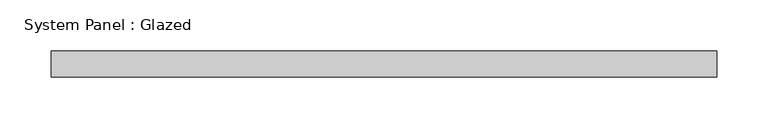
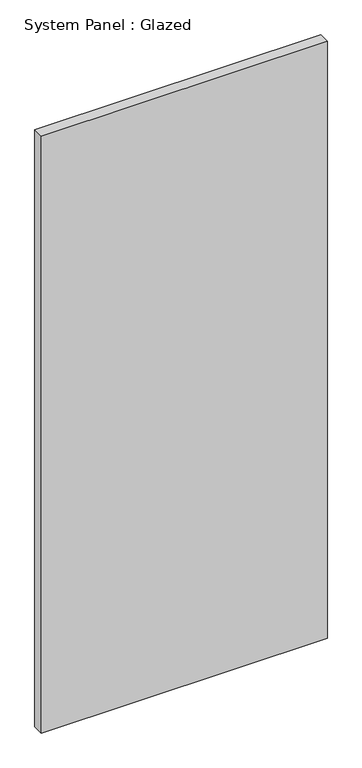
"""IFC4 building model written with IfcOpenShell, lengths in millimetres: plate geometry, System Panel : Glazed."""

from ifc_helpers import new_model, si_unit, origin, origin_with_axes, place, context, project, spatial, polyline, outline, extrude, source, transform, mapped, element, save


def system_panel_glazed_59bf60dd(model_context):
    return source(origin(), model_context, "Body", "SweptSolid", [
        extrude(outline(polyline([(323.85, 19.05), (-323.85, 19.05), (-323.85, 44.45), (323.85, 44.45), (323.85, 19.05)])), origin_with_axes(), (0.0, 0.0, 1.0), 1428.75),
    ])


if __name__ == "__main__":
    model = new_model("IFC4")
    model_context = context("Model", 3, world=origin())
    ifc_project = project(units=[si_unit("LENGTHUNIT", "METRE", prefix="MILLI")], contexts=[model_context])
    site = spatial("IfcSite", under=ifc_project)
    building = spatial("IfcBuilding", under=site)
    placement = place(None, origin())
    system_panel_glazed_shape = system_panel_glazed_59bf60dd(model_context)
    element("IfcPlate", 1, ObjectType="System Panel : Glazed", at=placement, inside=building, context=model_context, shape_type="MappedRepresentation", body=[
        mapped(system_panel_glazed_shape, transform((0.0, 0.0, 0.0), x_axis=(1.0, 0.0, 0.0), y_axis=(0.0, 1.0, 0.0), z_axis=(0.0, 0.0, 1.0))),
    ])
    save(model, "model.ifc")

# Revit data of these elements
# Type "System Panel : Glazed"
#   Construction Type Id = "GSP4R"
#   Analytic Construction = "1/8 in Pilkington single glazing"
#   Visual Light Transmittance = 0.9
#   Solar Heat Gain Coefficient = 0.86
#   Heat Transfer Coefficient (U) = 1.18115 BTU/(h·ft²·°F)
#   Define Thermal Properties by = 1
# Element 1 (IfcPlate, "System Panel : Glazed")
#   Materials on its faces: "Glass"
# Materials
#   "Glass": class "Glass", colour RGB 0 128 192, transparency 0.75, Description = "Soda Lime Glass", Cost = 0
